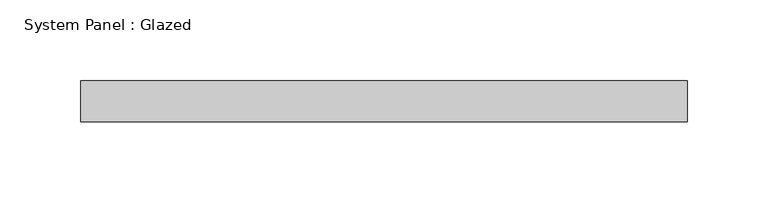
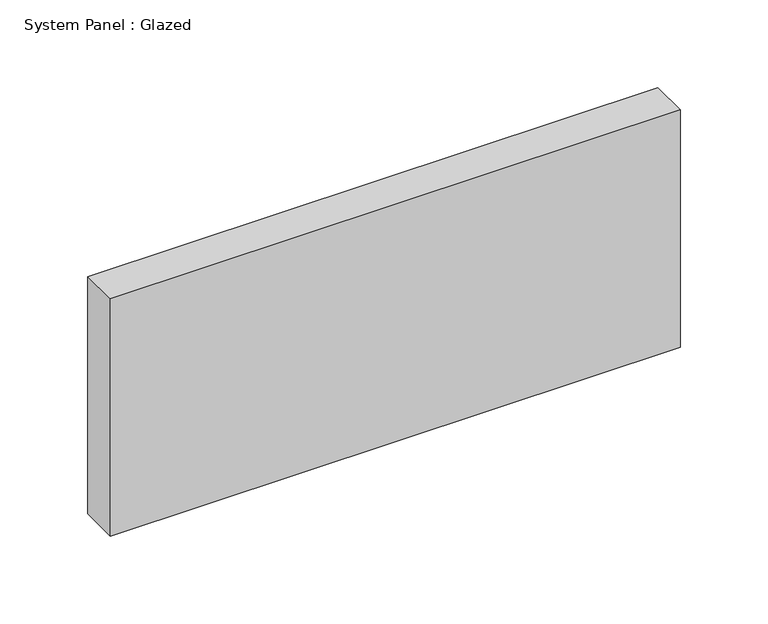
"""IFC4 building model written with IfcOpenShell, lengths in millimetres: plate geometry, System Panel : Glazed."""

from ifc_helpers import new_model, si_unit, origin, origin_with_axes, place, context, project, spatial, polyline, outline, extrude, source, transform, mapped, element, save


def system_panel_glazed_c4340a26(model_context):
    return source(origin(), model_context, "Body", "SweptSolid", [
        extrude(outline(polyline([(187.5766464, 19.05), (-187.5766464, 19.05), (-187.5766464, 44.45), (187.5766464, 44.45), (187.5766464, 19.05)])), origin_with_axes(), (0.0, 0.0, 1.0), 165.1),
    ])


if __name__ == "__main__":
    model = new_model("IFC4")
    model_context = context("Model", 3, world=origin())
    ifc_project = project(units=[si_unit("LENGTHUNIT", "METRE", prefix="MILLI")], contexts=[model_context])
    site = spatial("IfcSite", under=ifc_project)
    building = spatial("IfcBuilding", under=site)
    placement = place(None, origin())
    system_panel_glazed_shape = system_panel_glazed_c4340a26(model_context)
    element("IfcPlate", 1, ObjectType="System Panel : Glazed", at=placement, inside=building, context=model_context, shape_type="MappedRepresentation", body=[
        mapped(system_panel_glazed_shape, transform((0.0, 0.0, 0.0), x_axis=(1.0, 0.0, 0.0), y_axis=(0.0, 1.0, 0.0), z_axis=(0.0, 0.0, 1.0))),
    ])
    save(model, "model.ifc")

# Revit data of these elements
# Type "System Panel : Glazed"
#   Construction Type Id = "GSP4R"
#   Analytic Construction = "1/8 in Pilkington single glazing"
#   Visual Light Transmittance = 0.9
#   Solar Heat Gain Coefficient = 0.86
#   Heat Transfer Coefficient (U) = 1.18115 BTU/(h·ft²·°F)
#   Define Thermal Properties by = 1
# Element 1 (IfcPlate, "System Panel : Glazed")
#   Materials on its faces: "Glass"
# Materials
#   "Glass": class "Glass", colour RGB 0 128 192, transparency 0.75, Description = "Soda Lime Glass", Cost = 0
